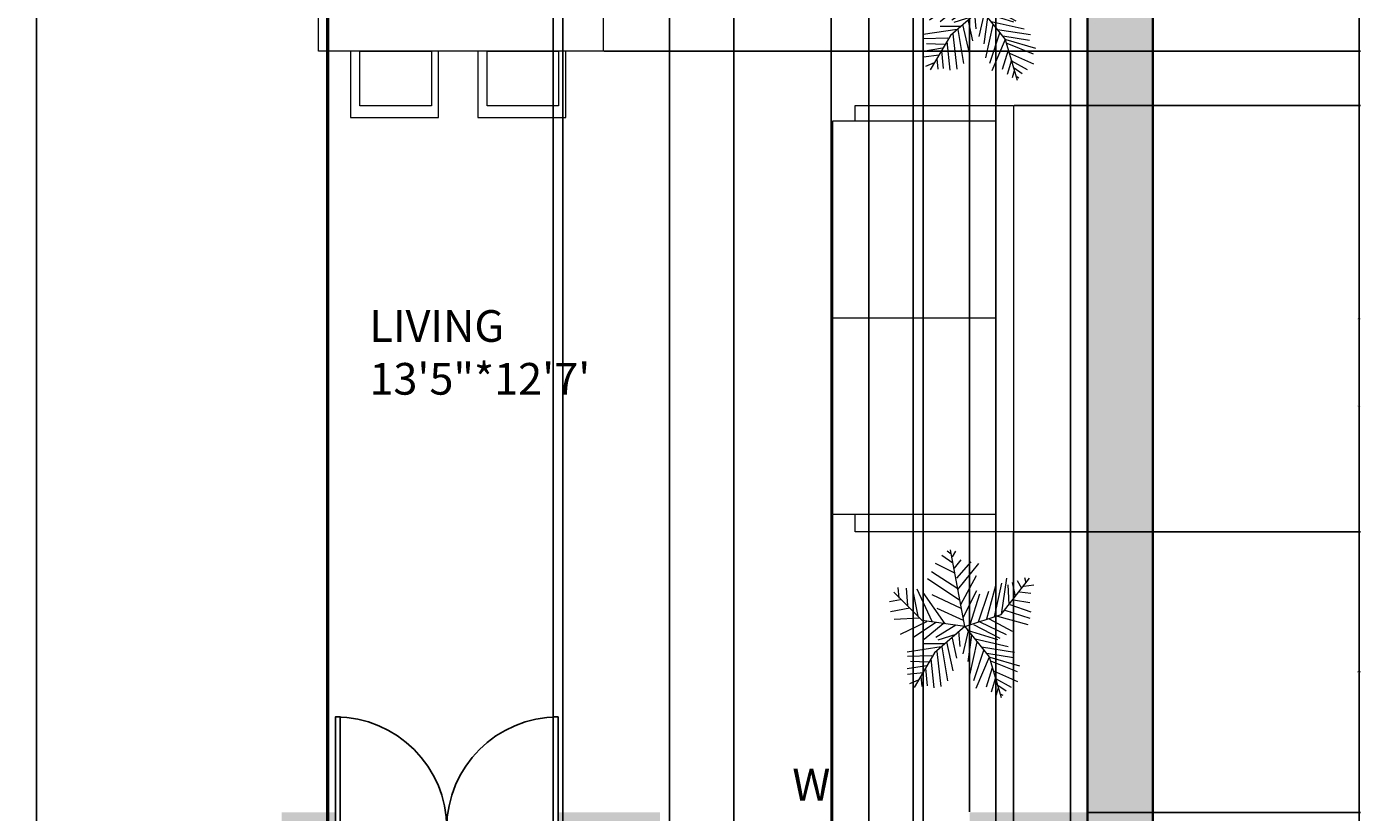
# Model space of a CAD drawing. Units: inches. Extents: x 2035 to 2384, y 1427 to 2020.
# Tile 4 of 7: x 2200 to 2383, y 1685 to 1794. Entities that reach past the tile are written whole.
import ezdxf

# ---------------------------------------------------------------- set-up
doc = ezdxf.new("R2010")
doc.units = ezdxf.units.IN
for name, color, linetype, lineweight in [('A-ANNO-DIMS', 2, 'Continuous', 18), ('A-ANNO-IDEN', 201, 'Continuous', 18), ('A-AREA-IDEN', 201, 'Continuous', 18), ('A-WALL-PATT', 140, 'Continuous', 13), ('C-PROP', 7, 'Continuous', 25), ('DOOR', 52, 'Continuous', 25), ('FUR', 71, 'Continuous', 18), ('L-PLNT', 112, 'Continuous', 18), ('WALL', 140, 'Continuous', 35)]:
    doc.layers.add(name, color=color, linetype=linetype, lineweight=lineweight)
doc.styles.get("Standard").update_dxf_attribs({"font": 'arial.ttf'})
doc.dimstyles.get("Standard").update_dxf_attribs({"dimtxt": 0.18, "dimasz": 0.18, "dimexe": 0.18, "dimexo": 0.0625, "dimgap": 0.09, "dimtad": 0, "dimtih": 1, "dimtoh": 1, "dimdec": 4, "dimzin": 0, "dimdsep": 46, "dimtxsty": 'Standard', "dimcen": 0.09, "dimadec": 0, "dimazin": 0, "dimtfac": 1, "dimtdec": 4, "dimtofl": 0, "dimtmove": 0, "dimatfit": 3, "dimfxl": 1, "dimtolj": 1, "dimtzin": 0, "dimarcsym": 0})

# ---------------------------------------------------------------- blocks, each defined once
blk = doc.blocks.new('*U2')
for p, q in [((0, 0), (0, -6)), ((40, 0), (40, -6))]:
    blk.add_line(p, q)
blk.add_lwpolyline([(0, 0), (0, 40), (1.75, 40), (1.75, 0)], close=True)
blk.add_arc((0, 0), 40, 0, 90)
blk = doc.blocks.new('*U6')
for p, q in [((-8.737, 47.138), (-17.069, 52.711)), ((-10.186, 53.64), (-13.084, 55.962)), ((0, 0), (-10.5, 57)), ((-9.099, 51.782), (-6.563, 55.962)), ((-7.65, 43.423), (-2.578, 49.46)), ((-5.114, 28.097), (-24.676, 40.636)), ((-7.288, 39.707), (-21.778, 46.673)), ((-5.839, 35.992), (4.667, 48.067)), ((-5.114, 27.632), (10.463, 46.673)), ((-3.665, 19.273), (-27.574, 35.527)), ((-2.941, 16.486), (8.652, 37.85)), ((16.259, 5.805), (23.142, 31.348)), ((22.055, 7.198), (27.489, 32.277)), ((27, 9), (48, 36)), ((27.127, 9.056), (31.112, 35.992)), ((31.836, 30.883), (32.561, 16.486)), ((35.096, 32.741), (37.27, 22.524)), ((38.719, 34.134), (41.979, 28.561)), ((43.791, 29.954), (51.036, 30.883)), ((44.153, 36.456), (45.239, 32.741)), ((-31.5, 4.5), (-52.5, 25.5)), ((-48.585, 21.131), (-49.309, 29.026)), ((-43.513, 28.561), (-42.427, 15.558)), ((-38.442, 26.239), (-34.819, 7.663)), ((-35.544, 28.097), (-24.314, 3.947)), ((-14.533, 2.09), (-30.834, 25.31)), ((-24.314, 23.917), (-2.941, 13.7)), ((-1.129, 6.734), (9.014, 26.704)), ((3.942, 1.625), (11.187, 24.381)), ((10.101, 3.483), (17.708, 26.239)), ((40.53, 25.775), (48.862, 24.846)), ((-47.498, 19.737), (-55.83, 18.344)), ((-40.615, 13.7), (-55.105, 10.913)), ((-20.691, 13.7), (-1.129, 4.876)), ((29.662, 12.307), (48.137, 6.269)), ((33.285, 16.486), (48.862, 10.913)), ((36.183, 19.737), (48.137, 17.88)), ((-33.37, 6.269), (-52.207, 5.34)), ((-28.299, 3.483), (-47.86, -5.805)), ((-21.416, 3.018), (-38.079, -8.128)), ((0, 0), (-31.5, 4.5)), ((-15.982, 2.09), (-30.11, -9.521)), ((0, 0), (-22.5, -19.5)), ((-6.563, 1.161), (-21.416, -8.128)), ((0, 0), (27, 9)), ((0, 0), (18, -22.5)), ((6.478, 1.625), (26.04, -8.592)), ((11.187, 3.483), (30.749, -5.805)), ((18.07, 5.805), (35.096, -3.483)), ((24.229, 7.663), (46.688, 1.625)), ((-6.563, -5.805), (-19.967, -9.985)), ((-9.461, -8.592), (-6.201, -23.453)), ((-4.752, -3.483), (-3.665, -14.629)), ((2.493, -3.019), (-1.491, -20.202)), ((1.769, -2.555), (24.229, -9.521)), ((5.029, -6.27), (2.131, -25.775)), ((7.565, -9.056), (32.198, -14.629)), ((-17.431, -15.094), (-42.789, -18.809)), ((-22.5, -19.5), (-37.5, -45)), ((-15.257, -12.772), (-30.11, -12.772)), ((-20.691, -18.345), (-17.793, -44.352)), ((-17.069, -15.094), (-12.721, -40.172)), ((-13.446, -11.378), (-8.737, -32.741)), ((9.014, -11.378), (3.58, -35.992)), ((14.085, -16.951), (6.478, -40.172)), ((12.274, -15.094), (36.907, -18.809)), ((16.259, -19.738), (36.183, -22.989)), ((-28.299, -29.026), (-42.789, -31.348)), ((-24.314, -21.596), (-42.427, -22.06)), ((-26.849, -26.24), (-40.253, -25.775)), ((-25.038, -23.918), (-22.865, -45.281)), ((18.07, -22.524), (8.289, -45.745)), ((18, -22.5), (27, -52.5)), ((18.433, -22.524), (40.53, -29.026)), ((19.157, -25.311), (38.719, -33.206)), ((-30.834, -34.135), (-42.427, -35.528)), ((-32.646, -36.921), (-31.921, -44.352)), ((-29.023, -30.884), (-27.936, -43.887)), ((20.244, -30.419), (15.897, -44.816)), ((22.78, -37.85), (19.519, -48.532)), ((21.331, -32.741), (39.081, -40.636)), ((22.78, -38.314), (34.372, -44.816)), ((-34.457, -39.708), (-40.978, -42.494)), ((24.591, -45.745), (23.142, -50.854)), ((24.591, -43.423), (30.749, -47.603)), ((26.764, -49.925), (28.213, -50.854))]:
    blk.add_line(p, q)
blk = doc.blocks.new('CHAIR-DINING')
for p, q in [((0, 0), (0, 9.14)), ((0, 9.14), (12.09, 9.14)), ((12.09, 9.14), (12.09, 0))]:
    blk.add_line(p, q)
blk.add_lwpolyline([(1.26, 0), (11.11, 0), (11.11, 7.54), (1.26, 7.54)], close=True)
blk = doc.blocks.new('*D23')
at = {"layer": 'A-ANNO-DIMS', "color": 0, "lineweight": -2, "transparency": 16777216}
for p, q in [((2354.82, 1981.38), (2383.33, 1981.38)), ((2383.15, 1981.2), (2383.15, 1741.56)), ((2383.15, 1501.56), (2383.15, 1741.2)), ((2354.82, 1501.38), (2383.33, 1501.38))]:
    blk.add_line(p, q, dxfattribs=at)
at = {"layer": 'A-ANNO-DIMS', "color": 0, "lineweight": 100, "transparency": 16777216}
for points in [[(2383.12, 1981.2), (2383.18, 1981.2), (2383.15, 1981.38)], [(2383.12, 1501.56), (2383.18, 1501.56), (2383.15, 1501.38)]]:
    blk.add_solid(points, dxfattribs=at)
at = {"layer": 'Defpoints', "color": 0, "lineweight": 100, "transparency": 16777216}
for p in [(2354.75, 1981.38), (2383.15, 1981.38), (2354.75, 1501.38)]:
    blk.add_point(p, dxfattribs=at)
at = {"layer": 'A-ANNO-DIMS', "color": 0, "transparency": 16777216, "insert": (2383.15, 1741.38), "char_height": 0.18, "attachment_point": 5}
blk.add_mtext('\\A1;480', dxfattribs=at)
blk = doc.blocks.new('*D25')
at = {"layer": 'A-ANNO-DIMS', "color": 0, "lineweight": -2, "transparency": 16777216}
for p, q in [((2241.25, 1503.69), (2241.25, 2009.96)), ((2241.43, 2009.78), (2256.26, 2009.78)), ((2272.01, 2009.78), (2257.18, 2009.78)), ((2272.19, 1503.69), (2272.19, 2009.96))]:
    blk.add_line(p, q, dxfattribs=at)
at = {"layer": 'A-ANNO-DIMS', "color": 0, "lineweight": 100, "transparency": 16777216}
for points in [[(2241.43, 2009.81), (2241.43, 2009.75), (2241.25, 2009.78)], [(2272.01, 2009.81), (2272.01, 2009.75), (2272.19, 2009.78)]]:
    blk.add_solid(points, dxfattribs=at)
at = {"layer": 'Defpoints', "color": 0, "lineweight": 100, "transparency": 16777216}
for p in [(2272.19, 2009.78), (2241.25, 1503.63), (2272.19, 1503.63)]:
    blk.add_point(p, dxfattribs=at)
at = {"layer": 'A-ANNO-DIMS', "color": 0, "transparency": 16777216, "insert": (2256.72, 2009.78), "char_height": 0.18, "attachment_point": 5}
blk.add_mtext('\\A1;30.935', dxfattribs=at)
blk = doc.blocks.new('*D26')
at = {"layer": 'A-ANNO-DIMS', "color": 0, "lineweight": -2, "transparency": 16777216}
for p, q in [((2272.19, 1506.56), (2272.19, 2009.96)), ((2272.37, 2009.78), (2297.26, 2009.78)), ((2322.93, 2009.78), (2298.04, 2009.78)), ((2323.11, 1506.56), (2323.11, 2009.96))]:
    blk.add_line(p, q, dxfattribs=at)
at = {"layer": 'A-ANNO-DIMS', "color": 0, "lineweight": 100, "transparency": 16777216}
for points in [[(2272.37, 2009.81), (2272.37, 2009.75), (2272.19, 2009.78)], [(2322.93, 2009.81), (2322.93, 2009.75), (2323.11, 2009.78)]]:
    blk.add_solid(points, dxfattribs=at)
at = {"layer": 'Defpoints', "color": 0, "lineweight": 100, "transparency": 16777216}
for p in [(2323.11, 2009.78), (2272.19, 1506.5), (2323.11, 1506.5)]:
    blk.add_point(p, dxfattribs=at)
at = {"layer": 'A-ANNO-DIMS', "color": 0, "transparency": 16777216, "insert": (2297.65, 2009.78), "char_height": 0.18, "attachment_point": 5}
blk.add_mtext('\\A1;50.92', dxfattribs=at)
blk = doc.blocks.new('*D40')
at = {"layer": 'A-ANNO-DIMS', "color": 0, "lineweight": -2, "transparency": 16777216}
for p, q in [((2201.01, 1835.82), (2201.01, 1427.17)), ((2241.01, 1835.82), (2241.01, 1427.17)), ((2201.19, 1427.35), (2220.79, 1427.35)), ((2240.83, 1427.35), (2221.24, 1427.35))]:
    blk.add_line(p, q, dxfattribs=at)
at = {"layer": 'A-ANNO-DIMS', "color": 0, "lineweight": 100, "transparency": 16777216}
for points in [[(2201.19, 1427.38), (2201.19, 1427.32), (2201.01, 1427.35)], [(2240.83, 1427.38), (2240.83, 1427.32), (2241.01, 1427.35)]]:
    blk.add_solid(points, dxfattribs=at)
at = {"layer": 'Defpoints', "color": 0, "lineweight": 100, "transparency": 16777216}
for p in [(2201.01, 1835.88), (2241.01, 1835.88), (2241.01, 1427.35)]:
    blk.add_point(p, dxfattribs=at)
at = {"layer": 'A-ANNO-DIMS', "color": 0, "transparency": 16777216, "insert": (2221.01, 1427.35), "char_height": 0.18, "attachment_point": 5}
blk.add_mtext('\\A1;40', dxfattribs=at)
blk = doc.blocks.new('*D41')
at = {"layer": 'A-ANNO-DIMS', "color": 0, "lineweight": -2, "transparency": 16777216}
for p, q in [((2273.51, 1840.32), (2273.51, 1427.17)), ((2310.46, 1840.32), (2310.46, 1427.17)), ((2273.69, 1427.35), (2291.59, 1427.35)), ((2310.28, 1427.35), (2292.38, 1427.35))]:
    blk.add_line(p, q, dxfattribs=at)
at = {"layer": 'A-ANNO-DIMS', "color": 0, "lineweight": 100, "transparency": 16777216}
for points in [[(2273.69, 1427.38), (2273.69, 1427.32), (2273.51, 1427.35)], [(2310.28, 1427.38), (2310.28, 1427.32), (2310.46, 1427.35)]]:
    blk.add_solid(points, dxfattribs=at)
at = {"layer": 'Defpoints', "color": 0, "lineweight": 100, "transparency": 16777216}
for p in [(2273.51, 1840.38), (2310.46, 1840.38), (2310.46, 1427.35)]:
    blk.add_point(p, dxfattribs=at)
at = {"layer": 'A-ANNO-DIMS', "color": 0, "transparency": 16777216, "insert": (2291.98, 1427.35), "char_height": 0.18, "attachment_point": 5}
blk.add_mtext('\\A1;36.95', dxfattribs=at)
blk = doc.blocks.new('*D42')
at = {"layer": 'A-ANNO-DIMS', "color": 0, "lineweight": -2, "transparency": 16777216}
for p, q in [((2297.05, 1925.82), (2297.05, 1427.17)), ((2333.11, 1925.82), (2333.11, 1427.17)), ((2297.23, 1427.35), (2314.69, 1427.35)), ((2332.93, 1427.35), (2315.47, 1427.35))]:
    blk.add_line(p, q, dxfattribs=at)
at = {"layer": 'A-ANNO-DIMS', "color": 0, "lineweight": 100, "transparency": 16777216}
for points in [[(2297.23, 1427.38), (2297.23, 1427.32), (2297.05, 1427.35)], [(2332.93, 1427.38), (2332.93, 1427.32), (2333.11, 1427.35)]]:
    blk.add_solid(points, dxfattribs=at)
at = {"layer": 'Defpoints', "color": 0, "lineweight": 100, "transparency": 16777216}
for p in [(2297.05, 1925.88), (2333.11, 1925.88), (2333.11, 1427.35)]:
    blk.add_point(p, dxfattribs=at)
at = {"layer": 'A-ANNO-DIMS', "color": 0, "transparency": 16777216, "insert": (2315.08, 1427.35), "char_height": 0.18, "attachment_point": 5}
blk.add_mtext('\\A1;36.06', dxfattribs=at)
blk = doc.blocks.new('*D45')
at = {"layer": 'A-ANNO-DIMS', "color": 0, "lineweight": -2, "transparency": 16777216}
for p, q in [((2321.75, 1840.32), (2321.75, 1427.17)), ((2345.75, 1840.32), (2345.75, 1427.17)), ((2321.93, 1427.35), (2333.53, 1427.35)), ((2345.57, 1427.35), (2333.97, 1427.35))]:
    blk.add_line(p, q, dxfattribs=at)
at = {"layer": 'A-ANNO-DIMS', "color": 0, "lineweight": 100, "transparency": 16777216}
for points in [[(2321.93, 1427.38), (2321.93, 1427.32), (2321.75, 1427.35)], [(2345.57, 1427.38), (2345.57, 1427.32), (2345.75, 1427.35)]]:
    blk.add_solid(points, dxfattribs=at)
at = {"layer": 'Defpoints', "color": 0, "lineweight": 100, "transparency": 16777216}
for p in [(2321.75, 1840.38), (2345.75, 1840.38), (2345.75, 1427.35)]:
    blk.add_point(p, dxfattribs=at)
at = {"layer": 'A-ANNO-DIMS', "color": 0, "transparency": 16777216, "insert": (2333.75, 1427.35), "char_height": 0.18, "attachment_point": 5}
blk.add_mtext('\\A1;24', dxfattribs=at)
blk = doc.blocks.new('*D46')
at = {"layer": 'A-ANNO-DIMS', "color": 0, "lineweight": -2, "transparency": 16777216}
for p, q in [((2288.19, 1905.68), (2288.19, 1427.17)), ((2315.66, 1905.68), (2315.66, 1427.17)), ((2288.37, 1427.35), (2301.53, 1427.35)), ((2315.48, 1427.35), (2302.32, 1427.35))]:
    blk.add_line(p, q, dxfattribs=at)
at = {"layer": 'A-ANNO-DIMS', "color": 0, "lineweight": 100, "transparency": 16777216}
for points in [[(2288.37, 1427.38), (2288.37, 1427.32), (2288.19, 1427.35)], [(2315.48, 1427.38), (2315.48, 1427.32), (2315.66, 1427.35)]]:
    blk.add_solid(points, dxfattribs=at)
at = {"layer": 'Defpoints', "color": 0, "lineweight": 100, "transparency": 16777216}
for p in [(2288.19, 1905.75), (2315.66, 1905.75), (2315.66, 1427.35)]:
    blk.add_point(p, dxfattribs=at)
at = {"layer": 'A-ANNO-DIMS', "color": 0, "transparency": 16777216, "insert": (2301.92, 1427.35), "char_height": 0.18, "attachment_point": 5}
blk.add_mtext('\\A1;27.47', dxfattribs=at)
blk = doc.blocks.new('*D48')
at = {"layer": 'A-ANNO-DIMS', "color": 0, "lineweight": -2, "transparency": 16777216}
for p, q in [((2323.12, 1858.3), (2323.12, 1427.17)), ((2343.42, 1858.3), (2343.42, 1427.17)), ((2323.3, 1427.35), (2332.81, 1427.35)), ((2343.24, 1427.35), (2333.74, 1427.35))]:
    blk.add_line(p, q, dxfattribs=at)
at = {"layer": 'A-ANNO-DIMS', "color": 0, "lineweight": 100, "transparency": 16777216}
for points in [[(2323.3, 1427.38), (2323.3, 1427.32), (2323.12, 1427.35)], [(2343.24, 1427.38), (2343.24, 1427.32), (2343.42, 1427.35)]]:
    blk.add_solid(points, dxfattribs=at)
at = {"layer": 'Defpoints', "color": 0, "lineweight": 100, "transparency": 16777216}
for p in [(2323.12, 1858.36), (2343.42, 1858.36), (2343.42, 1427.35)]:
    blk.add_point(p, dxfattribs=at)
at = {"layer": 'A-ANNO-DIMS', "color": 0, "transparency": 16777216, "insert": (2333.27, 1427.35), "char_height": 0.18, "attachment_point": 5}
blk.add_mtext('\\A1;20.302', dxfattribs=at)
blk = doc.blocks.new('*D55')
at = {"layer": 'A-ANNO-DIMS', "color": 0, "lineweight": -2, "transparency": 16777216}
for p, q in [((2279.13, 1811.24), (2383.33, 1811.24)), ((2383.15, 1811.06), (2383.15, 1800.94)), ((2383.15, 1790.46), (2383.15, 1800.57)), ((2279.13, 1790.28), (2383.33, 1790.28))]:
    blk.add_line(p, q, dxfattribs=at)
at = {"layer": 'A-ANNO-DIMS', "color": 0, "lineweight": 100, "transparency": 16777216}
for points in [[(2383.12, 1811.06), (2383.18, 1811.06), (2383.15, 1811.24)], [(2383.12, 1790.46), (2383.18, 1790.46), (2383.15, 1790.28)]]:
    blk.add_solid(points, dxfattribs=at)
at = {"layer": 'Defpoints', "color": 0, "lineweight": 100, "transparency": 16777216}
for p in [(2279.07, 1811.24), (2383.15, 1811.24), (2279.07, 1790.28)]:
    blk.add_point(p, dxfattribs=at)
at = {"layer": 'A-ANNO-DIMS', "color": 0, "transparency": 16777216, "insert": (2383.15, 1800.76), "char_height": 0.18, "attachment_point": 5}
blk.add_mtext('\\A1;20.96', dxfattribs=at)
blk = doc.blocks.new('*D56')
at = {"layer": 'A-ANNO-DIMS', "color": 0, "lineweight": -2, "transparency": 16777216}
for p, q in [((2335.64, 1782.76), (2383.33, 1782.76)), ((2383.15, 1782.58), (2383.15, 1753.58)), ((2383.15, 1724.21), (2383.15, 1753.21)), ((2335.64, 1724.03), (2383.33, 1724.03))]:
    blk.add_line(p, q, dxfattribs=at)
at = {"layer": 'A-ANNO-DIMS', "color": 0, "lineweight": 100, "transparency": 16777216}
for points in [[(2383.12, 1782.58), (2383.18, 1782.58), (2383.15, 1782.76)], [(2383.12, 1724.21), (2383.18, 1724.21), (2383.15, 1724.03)]]:
    blk.add_solid(points, dxfattribs=at)
at = {"layer": 'Defpoints', "color": 0, "lineweight": 100, "transparency": 16777216}
for p in [(2335.58, 1782.76), (2383.15, 1782.76), (2335.58, 1724.03)]:
    blk.add_point(p, dxfattribs=at)
at = {"layer": 'A-ANNO-DIMS', "color": 0, "transparency": 16777216, "insert": (2383.15, 1753.4), "char_height": 0.18, "attachment_point": 5}
blk.add_mtext('\\A1;58.73', dxfattribs=at)
blk = doc.blocks.new('*D57')
at = {"layer": 'A-ANNO-DIMS', "color": 0, "lineweight": -2, "transparency": 16777216}
for p, q in [((2310.65, 1726.38), (2310.65, 1427.17)), ((2335.58, 1723.97), (2335.58, 1427.17)), ((2310.83, 1427.35), (2322.65, 1427.35)), ((2335.4, 1427.35), (2323.58, 1427.35))]:
    blk.add_line(p, q, dxfattribs=at)
at = {"layer": 'A-ANNO-DIMS', "color": 0, "lineweight": 100, "transparency": 16777216}
for points in [[(2310.83, 1427.38), (2310.83, 1427.32), (2310.65, 1427.35)], [(2335.4, 1427.38), (2335.4, 1427.32), (2335.58, 1427.35)]]:
    blk.add_solid(points, dxfattribs=at)
at = {"layer": 'Defpoints', "color": 0, "lineweight": 100, "transparency": 16777216}
for p in [(2310.65, 1726.45), (2335.58, 1724.03), (2335.58, 1427.35)]:
    blk.add_point(p, dxfattribs=at)
at = {"layer": 'A-ANNO-DIMS', "color": 0, "transparency": 16777216, "insert": (2323.12, 1427.35), "char_height": 0.18, "attachment_point": 5}
blk.add_mtext('\\A1;24.924', dxfattribs=at)
blk = doc.blocks.new('*D64')
at = {"layer": 'A-ANNO-DIMS', "color": 0, "lineweight": -2, "transparency": 16777216}
for p, q in [((2335.58, 1723.97), (2335.58, 1427.17)), ((2345.75, 1685.32), (2345.75, 1427.17)), ((2335.76, 1427.35), (2340.21, 1427.35)), ((2345.57, 1427.35), (2341.12, 1427.35))]:
    blk.add_line(p, q, dxfattribs=at)
at = {"layer": 'A-ANNO-DIMS', "color": 0, "lineweight": 100, "transparency": 16777216}
for points in [[(2335.76, 1427.38), (2335.76, 1427.32), (2335.58, 1427.35)], [(2345.57, 1427.38), (2345.57, 1427.32), (2345.75, 1427.35)]]:
    blk.add_solid(points, dxfattribs=at)
at = {"layer": 'Defpoints', "color": 0, "lineweight": 100, "transparency": 16777216}
for p in [(2335.58, 1724.03), (2345.75, 1685.38), (2345.75, 1427.35)]:
    blk.add_point(p, dxfattribs=at)
at = {"layer": 'A-ANNO-DIMS', "color": 0, "transparency": 16777216, "insert": (2340.67, 1427.35), "char_height": 0.18, "attachment_point": 5}
blk.add_mtext('\\A1;10.174', dxfattribs=at)
blk = doc.blocks.new('*D65')
at = {"layer": 'A-ANNO-DIMS', "color": 0, "lineweight": -2, "transparency": 16777216}
for p, q in [((2335.64, 1724.03), (2383.33, 1724.03)), ((2383.15, 1723.85), (2383.15, 1704.89)), ((2383.15, 1685.56), (2383.15, 1704.52)), ((2345.82, 1685.38), (2383.33, 1685.38))]:
    blk.add_line(p, q, dxfattribs=at)
at = {"layer": 'A-ANNO-DIMS', "color": 0, "lineweight": 100, "transparency": 16777216}
for points in [[(2383.12, 1723.85), (2383.18, 1723.85), (2383.15, 1724.03)], [(2383.12, 1685.56), (2383.18, 1685.56), (2383.15, 1685.38)]]:
    blk.add_solid(points, dxfattribs=at)
at = {"layer": 'Defpoints', "color": 0, "lineweight": 100, "transparency": 16777216}
for p in [(2335.58, 1724.03), (2345.75, 1685.38), (2383.15, 1685.38)]:
    blk.add_point(p, dxfattribs=at)
at = {"layer": 'A-ANNO-DIMS', "color": 0, "transparency": 16777216, "insert": (2383.15, 1704.71), "char_height": 0.18, "attachment_point": 5}
blk.add_mtext('\\A1;38.65', dxfattribs=at)
blk = doc.blocks.new('*D68')
at = {"layer": 'A-ANNO-DIMS', "color": 0, "lineweight": -2, "transparency": 16777216}
for p, q in [((2329.51, 1685.44), (2329.51, 2009.96)), ((2329.69, 2009.78), (2337.25, 2009.78)), ((2345.57, 2009.78), (2338.02, 2009.78)), ((2345.75, 1685.44), (2345.75, 2009.96))]:
    blk.add_line(p, q, dxfattribs=at)
at = {"layer": 'A-ANNO-DIMS', "color": 0, "lineweight": 100, "transparency": 16777216}
for points in [[(2329.69, 2009.81), (2329.69, 2009.75), (2329.51, 2009.78)], [(2345.57, 2009.81), (2345.57, 2009.75), (2345.75, 2009.78)]]:
    blk.add_solid(points, dxfattribs=at)
at = {"layer": 'Defpoints', "color": 0, "lineweight": 100, "transparency": 16777216}
for p in [(2345.75, 2009.78), (2329.51, 1685.38), (2345.75, 1685.38)]:
    blk.add_point(p, dxfattribs=at)
at = {"layer": 'A-ANNO-DIMS', "color": 0, "transparency": 16777216, "insert": (2337.63, 2009.78), "char_height": 0.18, "attachment_point": 5}
blk.add_mtext('\\A1;16.24', dxfattribs=at)

msp = doc.modelspace()

# ---------------------------------------------------------------- hatches: boundary and pattern name
at = {"layer": 'A-WALL-PATT'}
h = msp.add_hatch(color=256, dxfattribs=at)
h.dxf.hatch_style = 1
h.paths.add_polyline_path([(2145.6215, 1981.3816), (2123.7529, 1981.3816), (2123.7529, 1972.3816), (2145.6215, 1972.3816)])
h.paths.add_polyline_path([(2354.7529, 1981.3816), (2209.3767, 1981.3816), (2209.3767, 1972.3816), (2354.7529, 1972.3816)])
h.paths.add_polyline_path([(2123.7529, 1981.3816), (2114.7529, 1981.3816), (2114.7529, 1505.8816), (2123.7529, 1505.8816)])
h.paths.add_polyline_path([(2248.2529, 1928.1316), (2243.7529, 1928.1316), (2243.7529, 1840.3816), (2248.2529, 1840.3816)])
h.paths.add_polyline_path([(2297.0514, 1930.3816), (2284.6994, 1930.3816), (2284.6994, 1925.8816), (2297.0514, 1925.8816)])
h.paths.add_polyline_path([(2345.7529, 1930.3816), (2333.1098, 1930.3816), (2333.1098, 1925.8816), (2345.7529, 1925.8816)])
h.paths.add_polyline_path([(2354.7529, 1972.3816), (2345.7529, 1972.3816), (2345.7529, 1501.3816), (2354.7529, 1501.3816)])
h.paths.add_polyline_path([(2188.2529, 1835.8816), (2183.7529, 1835.8816), (2183.7529, 1831.3677), (2184.207, 1831.3677), (2188.2529, 1831.3677)])
h.paths.add_polyline_path([(2188.2529, 1804.3949), (2184.207, 1804.3949), (2183.7529, 1804.3949), (2183.7529, 1685.3816), (2188.2529, 1685.3816)])
h.paths.add_polyline_path([(2273.5087, 1840.3816), (2241.0146, 1840.3816), (2241.0146, 1835.8816), (2273.5087, 1835.8816)])
h.paths.add_polyline_path([(2345.7529, 1840.3816), (2310.4577, 1840.3816), (2310.4577, 1835.8816), (2345.7529, 1835.8816)])
h.paths.add_polyline_path([(2161.9064, 1524.4315), (2196.2972, 1524.4315), (2196.2972, 1533.4306), (2161.9064, 1533.4306)], flags=9)
h.paths.add_polyline_path([(2279.3058, 1589.7515), (2308.9483, 1589.7515), (2308.9483, 1598.7506), (2279.3058, 1598.7506)], flags=9)
h.paths.add_polyline_path([(2242.9684, 1662.1655), (2279.0513, 1662.1655), (2279.0513, 1671.1647), (2242.9684, 1671.1647)], flags=9)
h.paths.add_polyline_path([(2154.6483, 1622.8242), (2195.1309, 1622.8242), (2195.1309, 1639.1195), (2154.6483, 1639.1195)], flags=9)
h.paths.add_polyline_path([(2138.8708, 1715.378), (2162.5199, 1715.378), (2162.5199, 1731.6734), (2138.8708, 1731.6734)], flags=9)
h.paths.add_polyline_path([(2135.5598, 1791.707), (2165.1993, 1791.707), (2165.1993, 1808.0024), (2135.5598, 1808.0024)], flags=9)
h.paths.add_polyline_path([(2245.1071, 1740.4502), (2279.0303, 1740.4502), (2279.0303, 1756.7455), (2245.1071, 1756.7455)], flags=9)
h.paths.add_polyline_path([(2284.7312, 1866.5552), (2313.6916, 1866.5552), (2313.6916, 1890.2034), (2284.7312, 1890.2034)], flags=9)
h.paths.add_polyline_path([(2139.9071, 1874.6496), (2173.8303, 1874.6496), (2173.8303, 1890.9449), (2139.9071, 1890.9449)], flags=9)
h = msp.add_hatch(color=256, dxfattribs=at)
h.dxf.hatch_style = 1
h.paths.add_polyline_path([(2236.7529, 1556.8816), (2209.3767, 1556.8816), (2209.3767, 1547.8816), (2236.7529, 1547.8816)])
h.paths.add_polyline_path([(2241.2529, 1680.8816), (2236.7529, 1680.8816), (2236.7529, 1547.8816), (2241.2529, 1547.8816)])
h.paths.add_polyline_path([(2241.2529, 1505.8816), (2114.7529, 1505.8816), (2114.7529, 1501.3816), (2241.2529, 1501.3816)])
h.paths.add_polyline_path([(2242.179, 1683.1823), (2242.179, 1685.3816), (2234.769, 1685.3816), (2234.769, 1680.8816), (2242.179, 1680.8816)])
h.paths.add_polyline_path([(2286.8795, 1685.3816), (2272.8549, 1685.3816), (2272.8549, 1683.1823), (2272.8549, 1680.8816), (2286.8795, 1680.8816)])
h.paths.add_polyline_path([(2345.7529, 1685.3816), (2329.513, 1685.3816), (2329.513, 1680.8816), (2345.7529, 1680.8816)])
h.paths.add_polyline_path([(2279.3058, 1589.7515), (2308.9483, 1589.7515), (2308.9483, 1598.7506), (2279.3058, 1598.7506)], flags=9)
h.paths.add_polyline_path([(2242.9684, 1662.1655), (2279.0513, 1662.1655), (2279.0513, 1671.1647), (2242.9684, 1671.1647)], flags=9)
h.paths.add_polyline_path([(2154.6483, 1622.8242), (2195.1309, 1622.8242), (2195.1309, 1639.1195), (2154.6483, 1639.1195)], flags=9)
h.paths.add_polyline_path([(2138.8708, 1715.378), (2162.5199, 1715.378), (2162.5199, 1731.6734), (2138.8708, 1731.6734)], flags=9)
h.paths.add_polyline_path([(2135.5598, 1791.707), (2165.1993, 1791.707), (2165.1993, 1808.0024), (2135.5598, 1808.0024)], flags=9)
h.paths.add_polyline_path([(2245.1071, 1740.4502), (2279.0303, 1740.4502), (2279.0303, 1756.7455), (2245.1071, 1756.7455)], flags=9)
h.paths.add_polyline_path([(2284.7312, 1866.5552), (2313.6916, 1866.5552), (2313.6916, 1890.2034), (2284.7312, 1890.2034)], flags=9)
h.paths.add_polyline_path([(2284.6985, 1943.1527), (2309.7208, 1943.1527), (2309.7208, 1959.448), (2284.6985, 1959.448)], flags=9)
h.paths.add_polyline_path([(2139.9071, 1874.6496), (2173.8303, 1874.6496), (2173.8303, 1890.9449), (2139.9071, 1890.9449)], flags=9)
h = msp.add_hatch(color=256, dxfattribs=at)
h.dxf.hatch_style = 1
h.paths.add_polyline_path([(2201.0146, 1840.3816), (2123.7529, 1840.3816), (2123.7529, 1835.8816), (2201.0146, 1835.8816)])
h.paths.add_polyline_path([(2136.2543, 1763.8816), (2123.7529, 1763.8816), (2123.7529, 1759.3816), (2136.2543, 1759.3816)])
h.paths.add_polyline_path([(2183.7529, 1763.8816), (2169.7769, 1763.8816), (2169.7769, 1759.3816), (2183.7529, 1759.3816)])
h.paths.add_polyline_path([(2152.8338, 1685.1369), (2152.8338, 1685.3816), (2123.7529, 1685.3816), (2123.7529, 1680.8816), (2152.8338, 1680.8816)])
h.paths.add_polyline_path([(2194.769, 1685.3816), (2181.2028, 1685.3816), (2181.2028, 1685.1369), (2181.2028, 1680.8816), (2194.769, 1680.8816)])
h.paths.add_polyline_path([(2145.6215, 1556.8816), (2123.7529, 1556.8816), (2123.7529, 1547.8816), (2145.6215, 1547.8816)])
h.paths.add_polyline_path([(2161.9064, 1524.4315), (2196.2972, 1524.4315), (2196.2972, 1533.4306), (2161.9064, 1533.4306)], flags=9)
h.paths.add_polyline_path([(2279.3058, 1589.7515), (2308.9483, 1589.7515), (2308.9483, 1598.7506), (2279.3058, 1598.7506)], flags=9)
h.paths.add_polyline_path([(2242.9684, 1662.1655), (2279.0513, 1662.1655), (2279.0513, 1671.1647), (2242.9684, 1671.1647)], flags=9)
h.paths.add_polyline_path([(2154.6483, 1622.8242), (2195.1309, 1622.8242), (2195.1309, 1639.1195), (2154.6483, 1639.1195)], flags=9)
h.paths.add_polyline_path([(2138.8708, 1715.378), (2162.5199, 1715.378), (2162.5199, 1731.6734), (2138.8708, 1731.6734)], flags=9)
h.paths.add_polyline_path([(2135.5598, 1791.707), (2165.1993, 1791.707), (2165.1993, 1808.0024), (2135.5598, 1808.0024)], flags=9)
h.paths.add_polyline_path([(2245.1071, 1740.4502), (2279.0303, 1740.4502), (2279.0303, 1756.7455), (2245.1071, 1756.7455)], flags=9)
h.paths.add_polyline_path([(2284.7312, 1866.5552), (2313.6916, 1866.5552), (2313.6916, 1890.2034), (2284.7312, 1890.2034)], flags=9)
h.paths.add_polyline_path([(2284.6985, 1943.1527), (2309.7208, 1943.1527), (2309.7208, 1959.448), (2284.6985, 1959.448)], flags=9)
h.paths.add_polyline_path([(2139.9071, 1874.6496), (2173.8303, 1874.6496), (2173.8303, 1890.9449), (2139.9071, 1890.9449)], flags=9)

# ---------------------------------------------------------------- linework, layer by layer
at = {"layer": 'C-PROP'}
msp.add_line((2354.7529, 1981.3816), (2354.7529, 1501.3816), dxfattribs=at)
msp.add_lwpolyline([(2114.7529, 1981.3816), (2354.7529, 1981.3816), (2354.7529, 1501.3816), (2114.7529, 1501.3816)], close=True, dxfattribs=at)
at = {"layer": 'FUR'}
for p, q in [((2313.7595, 1780.6044), (2313.7595, 1782.7604)), ((2313.7595, 1782.7604), (2335.5788, 1782.7604)), ((2335.5788, 1782.7604), (2335.5788, 1724.0323)), ((2310.655, 1753.5251), (2333.1419, 1753.5251)), ((2313.7595, 1724.0323), (2313.7595, 1726.4457)), ((2335.5788, 1724.0323), (2313.7595, 1724.0323))]:
    msp.add_line(p, q, dxfattribs=at)
for points in [[(2239.8773, 1811.2357), (2279.066, 1811.2357), (2279.066, 1790.2754), (2239.8773, 1790.2754)], [(2333.1419, 1780.6044), (2310.655, 1780.6044), (2310.655, 1726.4457), (2333.1419, 1726.4457)]]:
    msp.add_lwpolyline(points, close=True, dxfattribs=at)
at = {"layer": 'WALL'}
msp.add_lwpolyline([(2241.2529, 1552.3816), (2241.2529, 1505.8816), (2123.7529, 1505.8816), (2123.7529, 1972.3816), (2345.7529, 1972.3816), (2345.7529, 1503.6316), (2323.1125, 1503.6316)], dxfattribs=at)
msp.add_lwpolyline([(2345.7529, 1972.3816), (2354.7529, 1972.3816), (2354.7529, 1501.3816), (2345.7529, 1501.3816)], close=True, dxfattribs=at)

# ---------------------------------------------------------------- block references
at = {"layer": 'DOOR', "yscale": 0.3834481157981316, "zscale": 0.3834481157981316}
for p, xscale in [((2242.179, 1683.1823), 0.3834481157981316), ((2272.8549, 1683.1823), -0.3834481157981316)]:
    msp.add_blockref('*U2', p, dxfattribs=dict(at, xscale=xscale))
at = {"layer": 'FUR', "extrusion": (0, 0, -1), "zscale": -1, "rotation": 180}
for p in [(-2244.2838, 1790.2754), (-2261.8132, 1790.2754)]:
    msp.add_blockref('CHAIR-DINING', p, dxfattribs=at)
at = {"layer": 'L-PLNT', "xscale": 0.1859660506101331, "yscale": 0.1859660506101331, "zscale": 0.1859660506101331}
for p in [(2331.0601, 1796.0491), (2328.8554, 1710.9679)]:
    msp.add_blockref('*U6', p, dxfattribs=at)

# ---------------------------------------------------------------- texts
at = {"layer": 'A-ANNO-IDEN', "insert": (2305.1064, 1691.3746), "char_height": 4.367, "attachment_point": 1}
msp.add_mtext_dynamic_manual_height_columns('W', width=88.030619, gutter_width=21.835, heights=[0], dxfattribs=at)
at = {"layer": 'A-AREA-IDEN', "insert": (2246.8632, 1754.5754), "char_height": 4.366999, "attachment_point": 1}
msp.add_mtext_dynamic_manual_height_columns('LIVING\\P13\'5"*12\'7\'', width=88.030619, gutter_width=21.835, heights=[0], dxfattribs=at)

# ---------------------------------------------------------------- dimensions: what is measured, and where the dimension line sits
at = {"layer": 'A-ANNO-DIMS'}
for base, p1, p2, override, picture, middle in [((2272.1881, 2009.7816), (2241.2529, 1503.6316), (2272.1881, 1503.6316), {"dimdec": 3, "dimlfac": 1, "dimrnd": 0, "dimzin": 0, "dimdsep": 46, "dimlunit": 2}, '*D25', (2256.7205, 2009.7816)), ((2323.1125, 2009.7816), (2272.1881, 1506.4959), (2323.1125, 1506.4959), {"dimdec": 2, "dimlfac": 1, "dimrnd": 0, "dimzin": 0, "dimdsep": 46, "dimlunit": 2}, '*D26', (2297.6503, 2009.7816)), ((2345.7529, 2009.7816), (2329.513, 1685.3816), (2345.7529, 1685.3816), {"dimdec": 2, "dimlfac": 1, "dimrnd": 0, "dimzin": 0, "dimdsep": 46, "dimlunit": 2}, '*D68', (2337.633, 2009.7816)), ((2333.1098, 1427.3483), (2297.0514, 1925.8816), (2333.1098, 1925.8816), {"dimdec": 2, "dimlfac": 1, "dimrnd": 0, "dimzin": 0, "dimdsep": 46, "dimlunit": 2}, '*D42', (2315.0806, 1427.3483)), ((2315.6602, 1427.3483), (2288.1887, 1905.7459), (2315.6602, 1905.7459), {"dimdec": 2, "dimlfac": 1, "dimrnd": 0, "dimzin": 0, "dimdsep": 46, "dimlunit": 2}, '*D46', (2301.9245, 1427.3483)), ((2343.42295, 1427.348272), (2323.120454, 1858.361663), (2343.42295, 1858.361663), {"dimdec": 3, "dimlfac": 1, "dimrnd": 0, "dimzin": 0, "dimdsep": 46, "dimlunit": 2}, '*D48', (2333.271702, 1427.348272)), ((2310.4577, 1427.3483), (2273.5087, 1840.3816), (2310.4577, 1840.3816), {"dimdec": 2, "dimlfac": 1, "dimrnd": 0, "dimzin": 0, "dimdsep": 46, "dimlunit": 2}, '*D41', (2291.9832, 1427.3483)), ((2345.7529, 1427.3483), (2321.7529, 1840.3816), (2345.7529, 1840.3816), {"dimdec": 0, "dimlfac": 1, "dimrnd": 0, "dimzin": 0, "dimdsep": 46, "dimlunit": 2}, '*D45', (2333.7529, 1427.3483)), ((2241.0146, 1427.3483), (2201.0146, 1835.8816), (2241.0146, 1835.8816), {"dimdec": 0, "dimlfac": 1, "dimrnd": 0, "dimzin": 0, "dimdsep": 46, "dimlunit": 2}, '*D40', (2221.0146, 1427.3483)), ((2335.5788, 1427.3483), (2310.655, 1726.4457), (2335.5788, 1724.0323), {"dimdec": 3, "dimlfac": 1, "dimrnd": 0, "dimzin": 0, "dimdsep": 46, "dimlunit": 2}, '*D57', (2323.1169, 1427.3483)), ((2345.7529, 1427.3483), (2335.5788, 1724.0323), (2345.7529, 1685.3816), {"dimdec": 3, "dimlfac": 1, "dimrnd": 0, "dimzin": 0, "dimdsep": 46, "dimlunit": 2}, '*D64', (2340.6659, 1427.3483))]:
    dim = msp.add_linear_dim(base=base, p1=p1, p2=p2, dimstyle='Standard', override=override, dxfattribs=at)
    dim.commit()
    dim.dimension.update_dxf_attribs({"geometry": picture, "text_midpoint": middle})
for base, p1, p2, override, picture, middle in [((2383.1529, 1981.3816), (2354.7529, 1501.3816), (2354.7529, 1981.3816), {"dimdec": 0, "dimlfac": 1, "dimrnd": 0, "dimzin": 0, "dimdsep": 46, "dimlunit": 2}, '*D23', (2383.1529, 1741.3816)), ((2383.1529, 1811.2357), (2279.066, 1790.2754), (2279.066, 1811.2357), {"dimdec": 2, "dimlfac": 1, "dimrnd": 0, "dimzin": 0, "dimdsep": 46, "dimlunit": 2}, '*D55', (2383.1529, 1800.7556)), ((2383.1529, 1782.7604), (2335.5788, 1724.0323), (2335.5788, 1782.7604), {"dimdec": 2, "dimlfac": 1, "dimrnd": 0, "dimzin": 0, "dimdsep": 46, "dimlunit": 2}, '*D56', (2383.1529, 1753.3964)), ((2383.1529, 1685.3816), (2335.5788, 1724.0323), (2345.7529, 1685.3816), {"dimdec": 2, "dimlfac": 1, "dimrnd": 0, "dimzin": 0, "dimdsep": 46, "dimlunit": 2}, '*D65', (2383.1529, 1704.7069))]:
    dim = msp.add_linear_dim(base=base, p1=p1, p2=p2, angle=90, dimstyle='Standard', override=override, dxfattribs=at)
    dim.commit()
    dim.dimension.update_dxf_attribs({"geometry": picture, "text_midpoint": middle})

doc.saveas('drawing.dxf')
